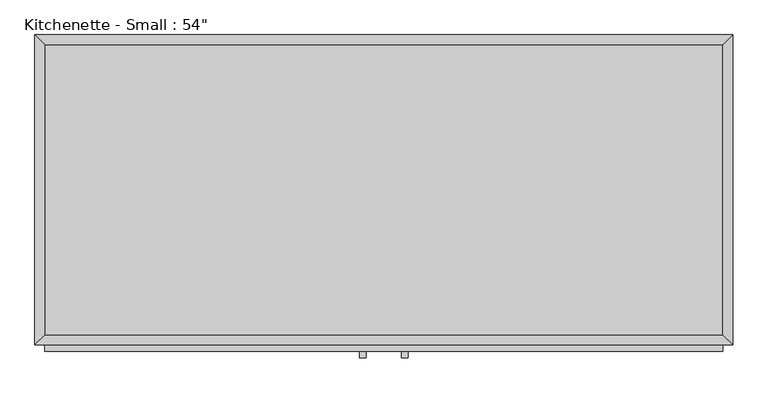
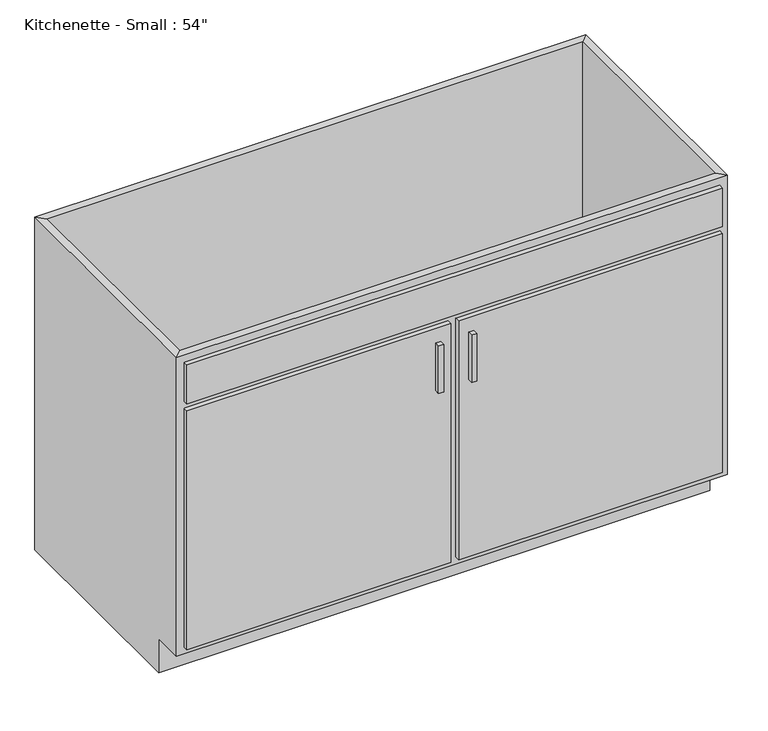
"""IFC4 building model written with IfcOpenShell, lengths in millimetres: proxy geometry."""

from ifc_helpers import new_model, si_unit, frame, origin, place, context, project, spatial, polyline, outline, extrude, faceted_brep, source, transform, mapped, element, save


def proxy_844211aa(model_context):
    return source(origin(), model_context, "Body", "SolidModel", [
        faceted_brep([(685.4877049, -590.55, 876.3), (685.4877049, -590.55, 88.9), (-648.0122951, -590.55, 88.9), (-648.0122951, -590.55, 876.3), (-667.0622951, -609.6, 876.3), (704.5377049, -609.6, 876.3), (-667.0622951, -609.6, 88.9), (704.5377049, -609.6, 88.9), (-648.0122951, -533.4, 88.9), (-648.0122951, -19.05, 88.9), (-648.0122951, -19.05, 876.3), (-667.0622951, 0.0, 876.3), (-667.0622951, 0.0, 0.0), (-667.0622951, -533.4, 0.0), (-667.0622951, -533.4, 88.9), (685.4877049, -19.05, 88.9), (685.4877049, -19.05, 876.3), (704.5377049, 0.0, 876.3), (704.5377049, 0.0, 0.0), (685.4877049, -533.4, 88.9), (704.5377049, -533.4, 88.9), (704.5377049, -533.4, 0.0)], [[[0, 1, 2, 3]], [[0, 3, 4, 5]], [[5, 4, 6, 7]], [[2, 1, 7, 6]], [[3, 2, 8, 9, 10]], [[4, 3, 10, 11]], [[6, 4, 11, 12, 13, 14]], [[2, 6, 14, 8]], [[10, 9, 15, 16]], [[11, 10, 16, 17]], [[12, 11, 17, 18]], [[1, 0, 16, 15, 19]], [[0, 5, 17, 16]], [[5, 7, 20, 21, 18, 17]], [[7, 1, 19, 20]], [[8, 19, 15, 9]], [[18, 21, 13, 12]], [[13, 21, 20, 19, 8, 14]]]),
        extrude(outline(polyline([(-16.1872951, -635.0), (-28.8872951, -635.0), (-28.8872951, -622.3), (-16.1872951, -622.3), (-16.1872951, -635.0)])), frame((0.0, 0.0, 573.769895), z_axis=(0.0, 0.0, 1.0), x_axis=(1.0, 0.0, 0.0)), (0.0, 0.0, 1.0), 124.730105),
        extrude(outline(polyline([(66.3627049, -635.0), (53.6627049, -635.0), (53.6627049, -622.3), (66.3627049, -622.3), (66.3627049, -635.0)])), frame((0.0, 0.0, 573.769895), z_axis=(0.0, 0.0, 1.0), x_axis=(1.0, 0.0, 0.0)), (0.0, 0.0, 1.0), 124.730105),
        extrude(outline(polyline([(685.4877049, -19.05), (685.4877049, -590.55), (-648.0122951, -590.55), (-648.0122951, -19.05), (685.4877049, -19.05)])), frame((0.0, 0.0, 88.9), z_axis=(0.0, 0.0, 1.0), x_axis=(1.0, 0.0, 0.0)), (0.0, 0.0, 1.0), 19.05),
        extrude(outline(polyline([(9.2127049, -622.3), (-648.0122951, -622.3), (-648.0122951, -609.6), (9.2127049, -609.6), (9.2127049, -622.3)])), frame((0.0, 0.0, 107.95), z_axis=(0.0, 0.0, 1.0), x_axis=(1.0, 0.0, 0.0)), (0.0, 0.0, 1.0), 628.65),
        extrude(outline(polyline([(685.4877049, -622.3), (28.2627049, -622.3), (28.2627049, -609.6), (685.4877049, -609.6), (685.4877049, -622.3)])), frame((0.0, 0.0, 107.95), z_axis=(0.0, 0.0, 1.0), x_axis=(1.0, 0.0, 0.0)), (0.0, 0.0, 1.0), 628.65),
        extrude(outline(polyline([(685.4877049, -622.3), (-648.0122951, -622.3), (-648.0122951, -609.6), (685.4877049, -609.6), (685.4877049, -622.3)])), frame((0.0, 0.0, 755.65), z_axis=(0.0, 0.0, 1.0), x_axis=(1.0, 0.0, 0.0)), (0.0, 0.0, 1.0), 101.6),
    ])


if __name__ == "__main__":
    model = new_model("IFC4")
    model_context = context("Model", 3, world=origin())
    ifc_project = project(units=[si_unit("LENGTHUNIT", "METRE", prefix="MILLI")], contexts=[model_context])
    site = spatial("IfcSite", under=ifc_project)
    building = spatial("IfcBuilding", under=site)
    placement = place(None, origin())
    proxy_shape = proxy_844211aa(model_context)
    element("IfcBuildingElementProxy", 1, Name="Kitchenette - Small : 54\"", ObjectType="Kitchenette - Small : 54\"", at=placement, inside=building, context=model_context, shape_type="MappedRepresentation", body=[
        mapped(proxy_shape, transform((0.0, 0.0, 0.0), x_axis=(1.0, 0.0, 0.0), y_axis=(0.0, 1.0, 0.0), z_axis=(0.0, 0.0, 1.0))),
    ])
    save(model, "model.ifc")

# Revit data of these elements
# Type "Kitchenette - Small : 54\""
#   Assembly Code = "E1090400"
#   Width = 4' - 6"
#   Height = 2' - 10 1/2"
#   Depth = 2' - 0"
#   Toe Depth = 0' - 3"
#   Toe Height = 0' - 3 1/2"
#   Cabinet Material = Cabinets
#   Door/Drawer Material = Cabinets
#   Handle Material = Cabinets - Handles
#   Default Elevation = 0
# Element 1 (IfcBuildingElementProxy, "Kitchenette - Small : 54\"")
#   Materials on its faces: "Cabinets", "Cabinets - Handles"
# Materials
#   "Cabinets": colour RGB 249 249 249, transparency 0
#   "Cabinets - Handles": class "Metal", colour RGB 57 57 57, transparency 0
